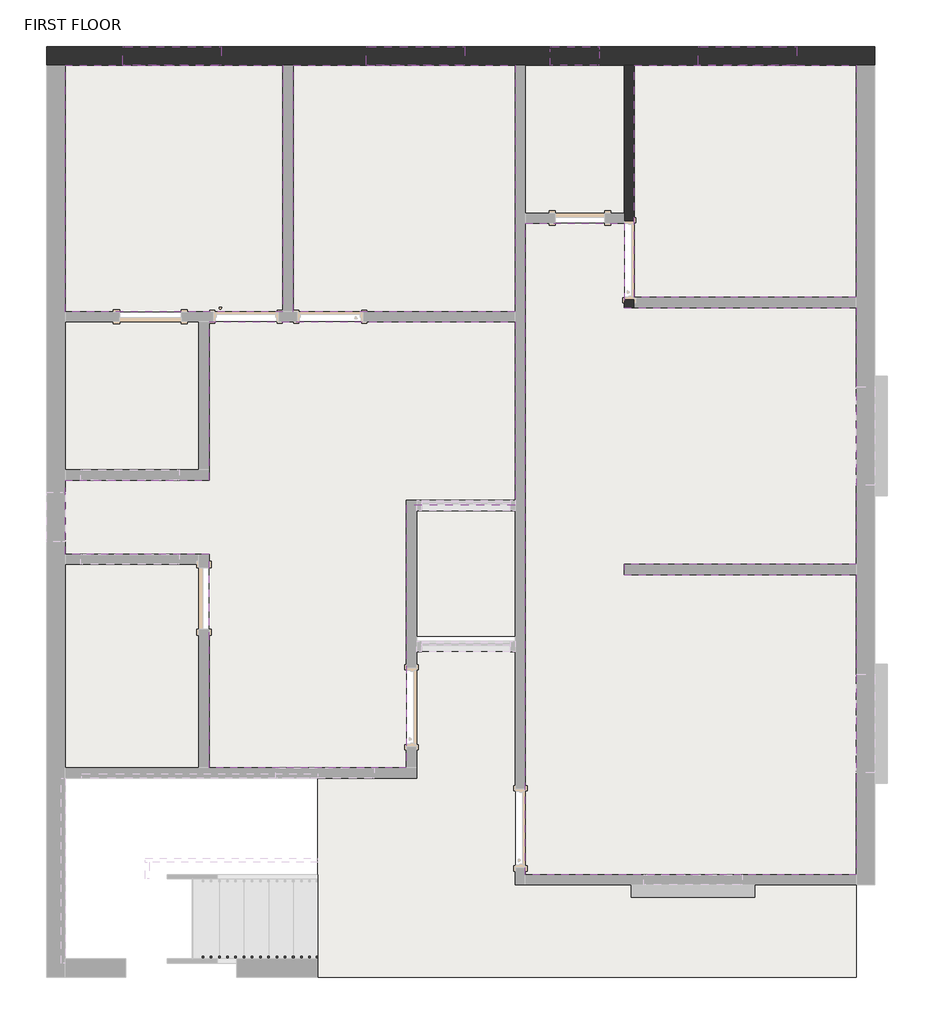
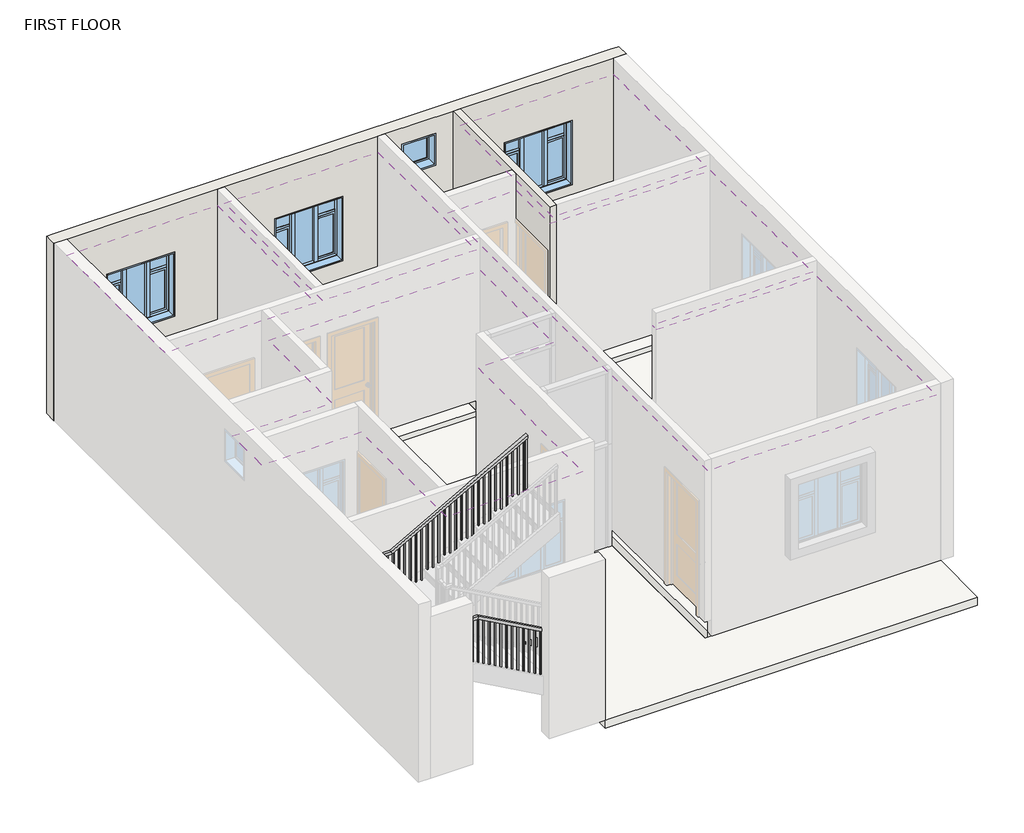
# One storey, part 2 of 3: 5 coverings, 4 windows, 2 walls, 1 railing, 1 slab.
"""IFC4 building model written with IfcOpenShell, lengths in millimetres."""

from ifc_helpers import new_model, si_unit, frame, origin, place, context, project, spatial, polyline, outline, extrude, faceted_brep, transform, mapped, element, save
from components import fixed_opening_window_2_x_2_e119d648, window_casement_triple_side_transom_window_4_x_4_fd24aed3

model = new_model("IFC4")

# Units and contexts
model_context = context("Model", 3, world=origin())
ifc_project = project(units=[si_unit("LENGTHUNIT", "METRE", prefix="MILLI")], contexts=[model_context])

# Site, building, storey
site = spatial("IfcSite", under=ifc_project)
building = spatial("IfcBuilding", under=site)
storey = spatial("IfcBuildingStorey", under=building, Name="FIRST FLOOR", Elevation=3352.8)

# Coverings
placement = place(None, origin())
element("IfcCovering", 1, ObjectType="GWB on Mtl. Stud 2", at=placement, inside=storey, context=model_context, shape_type="SweptSolid", body=[
    extrude(outline(polyline([(-14760.7023867, 8292.2500137), (-12068.3023867, 8292.2500137), (-12068.3023867, 5244.2500137), (-14760.7023867, 5244.2500137), (-14760.7023867, 8292.2500137)])), frame((0.0, 0.0, 6400.8), z_axis=(0.0, 0.0, 1.0), x_axis=(1.0, 0.0, 0.0)), (0.0, 0.0, 1.0), 107.95),
])
element("IfcCovering", 2, ObjectType="GWB on Mtl. Stud 2", at=placement, inside=storey, context=model_context, shape_type="SweptSolid", body=[
    extrude(outline(polyline([(-11941.3023867, 5244.2500137), (-11941.3023867, 8292.2500137), (-9198.1023867, 8292.2500137), (-9198.1023867, 5244.2500137), (-11941.3023867, 5244.2500137)])), frame((0.0, 0.0, 6400.8), z_axis=(0.0, 0.0, 1.0), x_axis=(1.0, 0.0, 0.0)), (0.0, 0.0, 1.0), 107.95),
])
element("IfcCovering", 3, ObjectType="GWB on Mtl. Stud 2", at=placement, inside=storey, context=model_context, shape_type="SweptSolid", body=[
    extrude(outline(polyline([(-7724.9023867, 5422.0500137), (-7724.9023867, 8292.2500137), (-4981.7023867, 8292.2500137), (-4981.7023867, 5422.0500137), (-7724.9023867, 5422.0500137)])), frame((0.0, 0.0, 6400.8), z_axis=(0.0, 0.0, 1.0), x_axis=(1.0, 0.0, 0.0)), (0.0, 0.0, 1.0), 107.95),
])
element("IfcCovering", 4, ObjectType="GWB on Mtl. Stud 2", at=placement, inside=storey, context=model_context, shape_type="SweptSolid", body=[
    extrude(outline(polyline([(-7851.9023867, 5295.0500137), (-4981.7023867, 5295.0500137), (-4981.7023867, 2120.0500137), (-7851.9023867, 2120.0500137), (-7851.9023867, 1993.0500137), (-4981.7023867, 1993.0500137), (-4981.7023867, -1715.3499863), (-9071.1023867, -1715.3499863), (-9071.1023867, 6336.4500137), (-7851.9023867, 6336.4500137), (-7851.9023867, 5295.0500137)])), frame((0.0, 0.0, 6400.8), z_axis=(0.0, 0.0, 1.0), x_axis=(1.0, 0.0, 0.0)), (0.0, 0.0, 1.0), 107.95),
])
element("IfcCovering", 5, ObjectType="GWB on Mtl. Stud 2", at=placement, inside=storey, context=model_context, shape_type="SweptSolid", body=[
    extrude(outline(polyline([(-12982.7023867, 2246.6265627), (-14760.7023867, 2246.6265627), (-14760.7023867, 3161.4500137), (-12982.7023867, 3161.4500137), (-12982.7023867, 5117.2500137), (-9198.1023867, 5117.2500137), (-9198.1023867, 2848.1833471), (-10544.3023867, 2848.1833471), (-10544.3023867, -394.5499863), (-12982.7023867, -394.5499863), (-12982.7023867, 2246.6265627)])), frame((0.0, 0.0, 6096.0), z_axis=(0.0, 0.0, 1.0), x_axis=(1.0, 0.0, 0.0)), (0.0, 0.0, 1.0), 107.95),
])

# Railing
element("IfcRailing", 6, ObjectType="Handrail - Rectangular", at=placement, inside=storey, context=model_context, shape_type="SolidModel", body=[
    faceted_brep([(-11636.5023867, -2756.7499863, 4741.3333333), (-11636.5023867, -2756.7499863, 4683.220221), (-11636.5023867, -2705.9499863, 4683.220221), (-11636.5023867, -2705.9499863, 4741.3333333), (-13770.1023867, -2756.7499863, 5926.6666667), (-13783.2659889, -2756.7499863, 5875.8666667), (-13783.2659889, -2705.9499863, 5875.8666667), (-13770.1023867, -2705.9499863, 5926.6666667), (-14760.7023867, -2756.7499863, 5926.6666667), (-14760.7023867, -2756.7499863, 5875.8666667), (-14709.9023867, -2705.9499863, 5875.8666667), (-14709.9023867, -2705.9499863, 5926.6666667), (-14760.7023867, -521.5499863, 5926.6666667), (-14760.7023867, -521.5499863, 5875.8666667), (-14709.9023867, -572.3499863, 5875.8666667), (-14709.9023867, -572.3499863, 5926.6666667), (-14074.9023867, -521.5499863, 5926.6666667), (-14061.7387844, -521.5499863, 5875.8666667), (-14061.7387844, -572.3499863, 5875.8666667), (-14074.9023867, -572.3499863, 5926.6666667), (-11636.5023867, -521.5499863, 7281.3333333), (-11636.5023867, -572.3499863, 7281.3333333), (-11636.5023867, -572.3499863, 7223.220221), (-11636.5023867, -521.5499863, 7223.220221)], [[[0, 1, 2, 3]], [[1, 0, 4, 5]], [[2, 1, 5, 6]], [[3, 2, 6, 7]], [[0, 3, 7, 4]], [[5, 4, 8, 9]], [[6, 5, 9, 10]], [[7, 6, 10, 11]], [[4, 7, 11, 8]], [[9, 8, 12, 13]], [[10, 9, 13, 14]], [[11, 10, 14, 15]], [[8, 11, 15, 12]], [[13, 12, 16, 17]], [[14, 13, 17, 18]], [[15, 14, 18, 19]], [[12, 15, 19, 16]], [[20, 21, 22, 23]], [[17, 16, 20, 23]], [[18, 17, 23, 22]], [[19, 18, 22, 21]], [[16, 19, 21, 20]]]),
    extrude(outline(polyline([(7189.7063321, -11696.8273867), (6197.6, -11696.8273867), (6197.6, -11677.7773867), (7200.2896654, -11677.7773867), (7189.7063321, -11696.8273867)])), frame((0.0, -556.4749863, 0.0), z_axis=(0.0, 1.0, 0.0), x_axis=(0.0, 0.0, 1.0)), (0.0, 0.0, 1.0), 19.05),
    extrude(outline(polyline([(7133.2618876, -11798.4273867), (6197.6, -11798.4273867), (6197.6, -11779.3773867), (7143.845221, -11779.3773867), (7133.2618876, -11798.4273867)])), frame((0.0, -556.4749863, 0.0), z_axis=(0.0, 1.0, 0.0), x_axis=(0.0, 0.0, 1.0)), (0.0, 0.0, 1.0), 19.05),
    extrude(outline(polyline([(7076.8174432, -11900.0273867), (6197.6, -11900.0273867), (6197.6, -11880.9773867), (7087.4007765, -11880.9773867), (7076.8174432, -11900.0273867)])), frame((0.0, -556.4749863, 0.0), z_axis=(0.0, 1.0, 0.0), x_axis=(0.0, 0.0, 1.0)), (0.0, 0.0, 1.0), 19.05),
    extrude(outline(polyline([(7020.3729988, -12001.6273867), (6028.2666667, -12001.6273867), (6028.2666667, -11982.5773867), (7030.9563321, -11982.5773867), (7020.3729988, -12001.6273867)])), frame((0.0, -556.4749863, 0.0), z_axis=(0.0, 1.0, 0.0), x_axis=(0.0, 0.0, 1.0)), (0.0, 0.0, 1.0), 19.05),
    extrude(outline(polyline([(6963.9285543, -12103.2273867), (6028.2666667, -12103.2273867), (6028.2666667, -12084.1773867), (6974.5118876, -12084.1773867), (6963.9285543, -12103.2273867)])), frame((0.0, -556.4749863, 0.0), z_axis=(0.0, 1.0, 0.0), x_axis=(0.0, 0.0, 1.0)), (0.0, 0.0, 1.0), 19.05),
    extrude(outline(polyline([(6907.4841099, -12204.8273867), (6028.2666667, -12204.8273867), (6028.2666667, -12185.7773867), (6918.0674432, -12185.7773867), (6907.4841099, -12204.8273867)])), frame((0.0, -556.4749863, 0.0), z_axis=(0.0, 1.0, 0.0), x_axis=(0.0, 0.0, 1.0)), (0.0, 0.0, 1.0), 19.05),
    extrude(outline(polyline([(6851.0396654, -12306.4273867), (5858.9333333, -12306.4273867), (5858.9333333, -12287.3773867), (6861.6229988, -12287.3773867), (6851.0396654, -12306.4273867)])), frame((0.0, -556.4749863, 0.0), z_axis=(0.0, 1.0, 0.0), x_axis=(0.0, 0.0, 1.0)), (0.0, 0.0, 1.0), 19.05),
    extrude(outline(polyline([(6794.595221, -12408.0273867), (5858.9333333, -12408.0273867), (5858.9333333, -12388.9773867), (6805.1785543, -12388.9773867), (6794.595221, -12408.0273867)])), frame((0.0, -556.4749863, 0.0), z_axis=(0.0, 1.0, 0.0), x_axis=(0.0, 0.0, 1.0)), (0.0, 0.0, 1.0), 19.05),
    extrude(outline(polyline([(6738.1507765, -12509.6273867), (5858.9333333, -12509.6273867), (5858.9333333, -12490.5773867), (6748.7341099, -12490.5773867), (6738.1507765, -12509.6273867)])), frame((0.0, -556.4749863, 0.0), z_axis=(0.0, 1.0, 0.0), x_axis=(0.0, 0.0, 1.0)), (0.0, 0.0, 1.0), 19.05),
    extrude(outline(polyline([(6681.7063321, -12611.2273867), (5689.6, -12611.2273867), (5689.6, -12592.1773867), (6692.2896654, -12592.1773867), (6681.7063321, -12611.2273867)])), frame((0.0, -556.4749863, 0.0), z_axis=(0.0, 1.0, 0.0), x_axis=(0.0, 0.0, 1.0)), (0.0, 0.0, 1.0), 19.05),
    extrude(outline(polyline([(6625.2618876, -12712.8273867), (5689.6, -12712.8273867), (5689.6, -12693.7773867), (6635.845221, -12693.7773867), (6625.2618876, -12712.8273867)])), frame((0.0, -556.4749863, 0.0), z_axis=(0.0, 1.0, 0.0), x_axis=(0.0, 0.0, 1.0)), (0.0, 0.0, 1.0), 19.05),
    extrude(outline(polyline([(6568.8174432, -12814.4273867), (5689.6, -12814.4273867), (5689.6, -12795.3773867), (6579.4007765, -12795.3773867), (6568.8174432, -12814.4273867)])), frame((0.0, -556.4749863, 0.0), z_axis=(0.0, 1.0, 0.0), x_axis=(0.0, 0.0, 1.0)), (0.0, 0.0, 1.0), 19.05),
    extrude(outline(polyline([(6512.3729988, -12916.0273867), (5520.2666667, -12916.0273867), (5520.2666667, -12896.9773867), (6522.9563321, -12896.9773867), (6512.3729988, -12916.0273867)])), frame((0.0, -556.4749863, 0.0), z_axis=(0.0, 1.0, 0.0), x_axis=(0.0, 0.0, 1.0)), (0.0, 0.0, 1.0), 19.05),
    extrude(outline(polyline([(6455.9285543, -13017.6273867), (5520.2666667, -13017.6273867), (5520.2666667, -12998.5773867), (6466.5118876, -12998.5773867), (6455.9285543, -13017.6273867)])), frame((0.0, -556.4749863, 0.0), z_axis=(0.0, 1.0, 0.0), x_axis=(0.0, 0.0, 1.0)), (0.0, 0.0, 1.0), 19.05),
    extrude(outline(polyline([(6399.4841099, -13119.2273867), (5520.2666667, -13119.2273867), (5520.2666667, -13100.1773867), (6410.0674432, -13100.1773867), (6399.4841099, -13119.2273867)])), frame((0.0, -556.4749863, 0.0), z_axis=(0.0, 1.0, 0.0), x_axis=(0.0, 0.0, 1.0)), (0.0, 0.0, 1.0), 19.05),
    extrude(outline(polyline([(6343.0396654, -13220.8273867), (5350.9333333, -13220.8273867), (5350.9333333, -13201.7773867), (6353.6229988, -13201.7773867), (6343.0396654, -13220.8273867)])), frame((0.0, -556.4749863, 0.0), z_axis=(0.0, 1.0, 0.0), x_axis=(0.0, 0.0, 1.0)), (0.0, 0.0, 1.0), 19.05),
    extrude(outline(polyline([(6286.595221, -13322.4273867), (5350.9333333, -13322.4273867), (5350.9333333, -13303.3773867), (6297.1785543, -13303.3773867), (6286.595221, -13322.4273867)])), frame((0.0, -556.4749863, 0.0), z_axis=(0.0, 1.0, 0.0), x_axis=(0.0, 0.0, 1.0)), (0.0, 0.0, 1.0), 19.05),
    extrude(outline(polyline([(6230.1507765, -13424.0273867), (5350.9333333, -13424.0273867), (5350.9333333, -13404.9773867), (6240.7341099, -13404.9773867), (6230.1507765, -13424.0273867)])), frame((0.0, -556.4749863, 0.0), z_axis=(0.0, 1.0, 0.0), x_axis=(0.0, 0.0, 1.0)), (0.0, 0.0, 1.0), 19.05),
    extrude(outline(polyline([(6173.7063321, -13525.6273867), (5181.6, -13525.6273867), (5181.6, -13506.5773867), (6184.2896654, -13506.5773867), (6173.7063321, -13525.6273867)])), frame((0.0, -556.4749863, 0.0), z_axis=(0.0, 1.0, 0.0), x_axis=(0.0, 0.0, 1.0)), (0.0, 0.0, 1.0), 19.05),
    extrude(outline(polyline([(6117.2618876, -13627.2273867), (5181.6, -13627.2273867), (5181.6, -13608.1773867), (6127.845221, -13608.1773867), (6117.2618876, -13627.2273867)])), frame((0.0, -556.4749863, 0.0), z_axis=(0.0, 1.0, 0.0), x_axis=(0.0, 0.0, 1.0)), (0.0, 0.0, 1.0), 19.05),
    extrude(outline(polyline([(6060.8174432, -13728.8273867), (5181.6, -13728.8273867), (5181.6, -13709.7773867), (6071.4007765, -13709.7773867), (6060.8174432, -13728.8273867)])), frame((0.0, -556.4749863, 0.0), z_axis=(0.0, 1.0, 0.0), x_axis=(0.0, 0.0, 1.0)), (0.0, 0.0, 1.0), 19.05),
    extrude(outline(polyline([(6004.3729988, -13830.4273867), (5012.2666667, -13830.4273867), (5012.2666667, -13811.3773867), (6014.9563321, -13811.3773867), (6004.3729988, -13830.4273867)])), frame((0.0, -556.4749863, 0.0), z_axis=(0.0, 1.0, 0.0), x_axis=(0.0, 0.0, 1.0)), (0.0, 0.0, 1.0), 19.05),
    extrude(outline(polyline([(5947.9285543, -13932.0273867), (5012.2666667, -13932.0273867), (5012.2666667, -13912.9773867), (5958.5118876, -13912.9773867), (5947.9285543, -13932.0273867)])), frame((0.0, -556.4749863, 0.0), z_axis=(0.0, 1.0, 0.0), x_axis=(0.0, 0.0, 1.0)), (0.0, 0.0, 1.0), 19.05),
    extrude(outline(polyline([(5891.4841099, -14033.6273867), (5012.2666667, -14033.6273867), (5012.2666667, -14014.5773867), (5902.0674432, -14014.5773867), (5891.4841099, -14033.6273867)])), frame((0.0, -556.4749863, 0.0), z_axis=(0.0, 1.0, 0.0), x_axis=(0.0, 0.0, 1.0)), (0.0, 0.0, 1.0), 19.05),
    extrude(outline(polyline([(-14135.2273867, -537.4249863), (-14116.1773867, -537.4249863), (-14116.1773867, -556.4749863), (-14135.2273867, -556.4749863), (-14135.2273867, -537.4249863)])), frame((0.0, 0.0, 5012.2666667), z_axis=(0.0, 0.0, 1.0), x_axis=(1.0, 0.0, 0.0)), (0.0, 0.0, 1.0), 863.6),
    extrude(outline(polyline([(-14236.8273867, -537.4249863), (-14217.7773867, -537.4249863), (-14217.7773867, -556.4749863), (-14236.8273867, -556.4749863), (-14236.8273867, -537.4249863)])), frame((0.0, 0.0, 5012.2666667), z_axis=(0.0, 0.0, 1.0), x_axis=(1.0, 0.0, 0.0)), (0.0, 0.0, 1.0), 863.6),
    extrude(outline(polyline([(-14338.4273867, -537.4249863), (-14319.3773867, -537.4249863), (-14319.3773867, -556.4749863), (-14338.4273867, -556.4749863), (-14338.4273867, -537.4249863)])), frame((0.0, 0.0, 5012.2666667), z_axis=(0.0, 0.0, 1.0), x_axis=(1.0, 0.0, 0.0)), (0.0, 0.0, 1.0), 863.6),
    extrude(outline(polyline([(-14440.0273867, -537.4249863), (-14420.9773867, -537.4249863), (-14420.9773867, -556.4749863), (-14440.0273867, -556.4749863), (-14440.0273867, -537.4249863)])), frame((0.0, 0.0, 5012.2666667), z_axis=(0.0, 0.0, 1.0), x_axis=(1.0, 0.0, 0.0)), (0.0, 0.0, 1.0), 863.6),
    extrude(outline(polyline([(-14541.6273867, -537.4249863), (-14522.5773867, -537.4249863), (-14522.5773867, -556.4749863), (-14541.6273867, -556.4749863), (-14541.6273867, -537.4249863)])), frame((0.0, 0.0, 5012.2666667), z_axis=(0.0, 0.0, 1.0), x_axis=(1.0, 0.0, 0.0)), (0.0, 0.0, 1.0), 863.6),
    extrude(outline(polyline([(-14643.2273867, -537.4249863), (-14624.1773867, -537.4249863), (-14624.1773867, -556.4749863), (-14643.2273867, -556.4749863), (-14643.2273867, -537.4249863)])), frame((0.0, 0.0, 5012.2666667), z_axis=(0.0, 0.0, 1.0), x_axis=(1.0, 0.0, 0.0)), (0.0, 0.0, 1.0), 863.6),
    extrude(outline(polyline([(-14744.8273867, -607.2749863), (-14744.8273867, -588.2249863), (-14725.7773867, -588.2249863), (-14725.7773867, -607.2749863), (-14744.8273867, -607.2749863)])), frame((0.0, 0.0, 5012.2666667), z_axis=(0.0, 0.0, 1.0), x_axis=(1.0, 0.0, 0.0)), (0.0, 0.0, 1.0), 863.6),
    extrude(outline(polyline([(-14744.8273867, -708.8749863), (-14744.8273867, -689.8249863), (-14725.7773867, -689.8249863), (-14725.7773867, -708.8749863), (-14744.8273867, -708.8749863)])), frame((0.0, 0.0, 5012.2666667), z_axis=(0.0, 0.0, 1.0), x_axis=(1.0, 0.0, 0.0)), (0.0, 0.0, 1.0), 863.6),
    extrude(outline(polyline([(-14744.8273867, -810.4749863), (-14744.8273867, -791.4249863), (-14725.7773867, -791.4249863), (-14725.7773867, -810.4749863), (-14744.8273867, -810.4749863)])), frame((0.0, 0.0, 5012.2666667), z_axis=(0.0, 0.0, 1.0), x_axis=(1.0, 0.0, 0.0)), (0.0, 0.0, 1.0), 863.6),
    extrude(outline(polyline([(-14744.8273867, -912.0749863), (-14744.8273867, -893.0249863), (-14725.7773867, -893.0249863), (-14725.7773867, -912.0749863), (-14744.8273867, -912.0749863)])), frame((0.0, 0.0, 5012.2666667), z_axis=(0.0, 0.0, 1.0), x_axis=(1.0, 0.0, 0.0)), (0.0, 0.0, 1.0), 863.6),
    extrude(outline(polyline([(-14744.8273867, -1013.6749863), (-14744.8273867, -994.6249863), (-14725.7773867, -994.6249863), (-14725.7773867, -1013.6749863), (-14744.8273867, -1013.6749863)])), frame((0.0, 0.0, 5012.2666667), z_axis=(0.0, 0.0, 1.0), x_axis=(1.0, 0.0, 0.0)), (0.0, 0.0, 1.0), 863.6),
    extrude(outline(polyline([(-14744.8273867, -1115.2749863), (-14744.8273867, -1096.2249863), (-14725.7773867, -1096.2249863), (-14725.7773867, -1115.2749863), (-14744.8273867, -1115.2749863)])), frame((0.0, 0.0, 5012.2666667), z_axis=(0.0, 0.0, 1.0), x_axis=(1.0, 0.0, 0.0)), (0.0, 0.0, 1.0), 863.6),
    extrude(outline(polyline([(-14744.8273867, -1216.8749863), (-14744.8273867, -1197.8249863), (-14725.7773867, -1197.8249863), (-14725.7773867, -1216.8749863), (-14744.8273867, -1216.8749863)])), frame((0.0, 0.0, 5012.2666667), z_axis=(0.0, 0.0, 1.0), x_axis=(1.0, 0.0, 0.0)), (0.0, 0.0, 1.0), 863.6),
    extrude(outline(polyline([(-14744.8273867, -1318.4749863), (-14744.8273867, -1299.4249863), (-14725.7773867, -1299.4249863), (-14725.7773867, -1318.4749863), (-14744.8273867, -1318.4749863)])), frame((0.0, 0.0, 5012.2666667), z_axis=(0.0, 0.0, 1.0), x_axis=(1.0, 0.0, 0.0)), (0.0, 0.0, 1.0), 863.6),
    extrude(outline(polyline([(-14744.8273867, -1420.0749863), (-14744.8273867, -1401.0249863), (-14725.7773867, -1401.0249863), (-14725.7773867, -1420.0749863), (-14744.8273867, -1420.0749863)])), frame((0.0, 0.0, 5012.2666667), z_axis=(0.0, 0.0, 1.0), x_axis=(1.0, 0.0, 0.0)), (0.0, 0.0, 1.0), 863.6),
    extrude(outline(polyline([(-14744.8273867, -1521.6749863), (-14744.8273867, -1502.6249863), (-14725.7773867, -1502.6249863), (-14725.7773867, -1521.6749863), (-14744.8273867, -1521.6749863)])), frame((0.0, 0.0, 5012.2666667), z_axis=(0.0, 0.0, 1.0), x_axis=(1.0, 0.0, 0.0)), (0.0, 0.0, 1.0), 863.6),
    extrude(outline(polyline([(-14744.8273867, -1623.2749863), (-14744.8273867, -1604.2249863), (-14725.7773867, -1604.2249863), (-14725.7773867, -1623.2749863), (-14744.8273867, -1623.2749863)])), frame((0.0, 0.0, 5012.2666667), z_axis=(0.0, 0.0, 1.0), x_axis=(1.0, 0.0, 0.0)), (0.0, 0.0, 1.0), 863.6),
    extrude(outline(polyline([(-14744.8273867, -1724.8749863), (-14744.8273867, -1705.8249863), (-14725.7773867, -1705.8249863), (-14725.7773867, -1724.8749863), (-14744.8273867, -1724.8749863)])), frame((0.0, 0.0, 5012.2666667), z_axis=(0.0, 0.0, 1.0), x_axis=(1.0, 0.0, 0.0)), (0.0, 0.0, 1.0), 863.6),
    extrude(outline(polyline([(-14744.8273867, -1826.4749863), (-14744.8273867, -1807.4249863), (-14725.7773867, -1807.4249863), (-14725.7773867, -1826.4749863), (-14744.8273867, -1826.4749863)])), frame((0.0, 0.0, 5012.2666667), z_axis=(0.0, 0.0, 1.0), x_axis=(1.0, 0.0, 0.0)), (0.0, 0.0, 1.0), 863.6),
    extrude(outline(polyline([(-14744.8273867, -1928.0749863), (-14744.8273867, -1909.0249863), (-14725.7773867, -1909.0249863), (-14725.7773867, -1928.0749863), (-14744.8273867, -1928.0749863)])), frame((0.0, 0.0, 5012.2666667), z_axis=(0.0, 0.0, 1.0), x_axis=(1.0, 0.0, 0.0)), (0.0, 0.0, 1.0), 863.6),
    extrude(outline(polyline([(-14744.8273867, -2029.6749863), (-14744.8273867, -2010.6249863), (-14725.7773867, -2010.6249863), (-14725.7773867, -2029.6749863), (-14744.8273867, -2029.6749863)])), frame((0.0, 0.0, 5012.2666667), z_axis=(0.0, 0.0, 1.0), x_axis=(1.0, 0.0, 0.0)), (0.0, 0.0, 1.0), 863.6),
    extrude(outline(polyline([(-14744.8273867, -2131.2749863), (-14744.8273867, -2112.2249863), (-14725.7773867, -2112.2249863), (-14725.7773867, -2131.2749863), (-14744.8273867, -2131.2749863)])), frame((0.0, 0.0, 5012.2666667), z_axis=(0.0, 0.0, 1.0), x_axis=(1.0, 0.0, 0.0)), (0.0, 0.0, 1.0), 863.6),
    extrude(outline(polyline([(-14744.8273867, -2232.8749863), (-14744.8273867, -2213.8249863), (-14725.7773867, -2213.8249863), (-14725.7773867, -2232.8749863), (-14744.8273867, -2232.8749863)])), frame((0.0, 0.0, 5012.2666667), z_axis=(0.0, 0.0, 1.0), x_axis=(1.0, 0.0, 0.0)), (0.0, 0.0, 1.0), 863.6),
    extrude(outline(polyline([(-14744.8273867, -2334.4749863), (-14744.8273867, -2315.4249863), (-14725.7773867, -2315.4249863), (-14725.7773867, -2334.4749863), (-14744.8273867, -2334.4749863)])), frame((0.0, 0.0, 5012.2666667), z_axis=(0.0, 0.0, 1.0), x_axis=(1.0, 0.0, 0.0)), (0.0, 0.0, 1.0), 863.6),
    extrude(outline(polyline([(-14744.8273867, -2436.0749863), (-14744.8273867, -2417.0249863), (-14725.7773867, -2417.0249863), (-14725.7773867, -2436.0749863), (-14744.8273867, -2436.0749863)])), frame((0.0, 0.0, 5012.2666667), z_axis=(0.0, 0.0, 1.0), x_axis=(1.0, 0.0, 0.0)), (0.0, 0.0, 1.0), 863.6),
    extrude(outline(polyline([(-14744.8273867, -2537.6749863), (-14744.8273867, -2518.6249863), (-14725.7773867, -2518.6249863), (-14725.7773867, -2537.6749863), (-14744.8273867, -2537.6749863)])), frame((0.0, 0.0, 5012.2666667), z_axis=(0.0, 0.0, 1.0), x_axis=(1.0, 0.0, 0.0)), (0.0, 0.0, 1.0), 863.6),
    extrude(outline(polyline([(-14744.8273867, -2639.2749863), (-14744.8273867, -2620.2249863), (-14725.7773867, -2620.2249863), (-14725.7773867, -2639.2749863), (-14744.8273867, -2639.2749863)])), frame((0.0, 0.0, 5012.2666667), z_axis=(0.0, 0.0, 1.0), x_axis=(1.0, 0.0, 0.0)), (0.0, 0.0, 1.0), 863.6),
    extrude(outline(polyline([(-14674.9773867, -2740.8749863), (-14694.0273867, -2740.8749863), (-14694.0273867, -2721.8249863), (-14674.9773867, -2721.8249863), (-14674.9773867, -2740.8749863)])), frame((0.0, 0.0, 5012.2666667), z_axis=(0.0, 0.0, 1.0), x_axis=(1.0, 0.0, 0.0)), (0.0, 0.0, 1.0), 863.6),
    extrude(outline(polyline([(-14573.3773867, -2740.8749863), (-14592.4273867, -2740.8749863), (-14592.4273867, -2721.8249863), (-14573.3773867, -2721.8249863), (-14573.3773867, -2740.8749863)])), frame((0.0, 0.0, 5012.2666667), z_axis=(0.0, 0.0, 1.0), x_axis=(1.0, 0.0, 0.0)), (0.0, 0.0, 1.0), 863.6),
    extrude(outline(polyline([(-14471.7773867, -2740.8749863), (-14490.8273867, -2740.8749863), (-14490.8273867, -2721.8249863), (-14471.7773867, -2721.8249863), (-14471.7773867, -2740.8749863)])), frame((0.0, 0.0, 5012.2666667), z_axis=(0.0, 0.0, 1.0), x_axis=(1.0, 0.0, 0.0)), (0.0, 0.0, 1.0), 863.6),
    extrude(outline(polyline([(-14370.1773867, -2740.8749863), (-14389.2273867, -2740.8749863), (-14389.2273867, -2721.8249863), (-14370.1773867, -2721.8249863), (-14370.1773867, -2740.8749863)])), frame((0.0, 0.0, 5012.2666667), z_axis=(0.0, 0.0, 1.0), x_axis=(1.0, 0.0, 0.0)), (0.0, 0.0, 1.0), 863.6),
    extrude(outline(polyline([(-14268.5773867, -2740.8749863), (-14287.6273867, -2740.8749863), (-14287.6273867, -2721.8249863), (-14268.5773867, -2721.8249863), (-14268.5773867, -2740.8749863)])), frame((0.0, 0.0, 5012.2666667), z_axis=(0.0, 0.0, 1.0), x_axis=(1.0, 0.0, 0.0)), (0.0, 0.0, 1.0), 863.6),
    extrude(outline(polyline([(-14166.9773867, -2740.8749863), (-14186.0273867, -2740.8749863), (-14186.0273867, -2721.8249863), (-14166.9773867, -2721.8249863), (-14166.9773867, -2740.8749863)])), frame((0.0, 0.0, 5012.2666667), z_axis=(0.0, 0.0, 1.0), x_axis=(1.0, 0.0, 0.0)), (0.0, 0.0, 1.0), 863.6),
    extrude(outline(polyline([(-14065.3773867, -2740.8749863), (-14084.4273867, -2740.8749863), (-14084.4273867, -2721.8249863), (-14065.3773867, -2721.8249863), (-14065.3773867, -2740.8749863)])), frame((0.0, 0.0, 5012.2666667), z_axis=(0.0, 0.0, 1.0), x_axis=(1.0, 0.0, 0.0)), (0.0, 0.0, 1.0), 863.6),
    extrude(outline(polyline([(-13963.7773867, -2740.8749863), (-13982.8273867, -2740.8749863), (-13982.8273867, -2721.8249863), (-13963.7773867, -2721.8249863), (-13963.7773867, -2740.8749863)])), frame((0.0, 0.0, 5012.2666667), z_axis=(0.0, 0.0, 1.0), x_axis=(1.0, 0.0, 0.0)), (0.0, 0.0, 1.0), 863.6),
    extrude(outline(polyline([(-13862.1773867, -2740.8749863), (-13881.2273867, -2740.8749863), (-13881.2273867, -2721.8249863), (-13862.1773867, -2721.8249863), (-13862.1773867, -2740.8749863)])), frame((0.0, 0.0, 5012.2666667), z_axis=(0.0, 0.0, 1.0), x_axis=(1.0, 0.0, 0.0)), (0.0, 0.0, 1.0), 863.6),
    extrude(outline(polyline([(5873.845221, -13779.6273867), (5012.2666667, -13779.6273867), (5012.2666667, -13760.5773867), (5863.2618876, -13760.5773867), (5873.845221, -13779.6273867)])), frame((0.0, -2740.8749863, 0.0), z_axis=(0.0, 1.0, 0.0), x_axis=(0.0, 0.0, 1.0)), (0.0, 0.0, 1.0), 19.05),
    extrude(outline(polyline([(5817.4007765, -13678.0273867), (4842.9333333, -13678.0273867), (4842.9333333, -13658.9773867), (5806.8174432, -13658.9773867), (5817.4007765, -13678.0273867)])), frame((0.0, -2740.8749863, 0.0), z_axis=(0.0, 1.0, 0.0), x_axis=(0.0, 0.0, 1.0)), (0.0, 0.0, 1.0), 19.05),
    extrude(outline(polyline([(5760.9563321, -13576.4273867), (4842.9333333, -13576.4273867), (4842.9333333, -13557.3773867), (5750.3729988, -13557.3773867), (5760.9563321, -13576.4273867)])), frame((0.0, -2740.8749863, 0.0), z_axis=(0.0, 1.0, 0.0), x_axis=(0.0, 0.0, 1.0)), (0.0, 0.0, 1.0), 19.05),
    extrude(outline(polyline([(5704.5118876, -13474.8273867), (4842.9333333, -13474.8273867), (4842.9333333, -13455.7773867), (5693.9285543, -13455.7773867), (5704.5118876, -13474.8273867)])), frame((0.0, -2740.8749863, 0.0), z_axis=(0.0, 1.0, 0.0), x_axis=(0.0, 0.0, 1.0)), (0.0, 0.0, 1.0), 19.05),
    extrude(outline(polyline([(5648.0674432, -13373.2273867), (4673.6, -13373.2273867), (4673.6, -13354.1773867), (5637.4841099, -13354.1773867), (5648.0674432, -13373.2273867)])), frame((0.0, -2740.8749863, 0.0), z_axis=(0.0, 1.0, 0.0), x_axis=(0.0, 0.0, 1.0)), (0.0, 0.0, 1.0), 19.05),
    extrude(outline(polyline([(5591.6229988, -13271.6273867), (4673.6, -13271.6273867), (4673.6, -13252.5773867), (5581.0396654, -13252.5773867), (5591.6229988, -13271.6273867)])), frame((0.0, -2740.8749863, 0.0), z_axis=(0.0, 1.0, 0.0), x_axis=(0.0, 0.0, 1.0)), (0.0, 0.0, 1.0), 19.05),
    extrude(outline(polyline([(5535.1785543, -13170.0273867), (4673.6, -13170.0273867), (4673.6, -13150.9773867), (5524.595221, -13150.9773867), (5535.1785543, -13170.0273867)])), frame((0.0, -2740.8749863, 0.0), z_axis=(0.0, 1.0, 0.0), x_axis=(0.0, 0.0, 1.0)), (0.0, 0.0, 1.0), 19.05),
    extrude(outline(polyline([(5478.7341099, -13068.4273867), (4504.2666667, -13068.4273867), (4504.2666667, -13049.3773867), (5468.1507765, -13049.3773867), (5478.7341099, -13068.4273867)])), frame((0.0, -2740.8749863, 0.0), z_axis=(0.0, 1.0, 0.0), x_axis=(0.0, 0.0, 1.0)), (0.0, 0.0, 1.0), 19.05),
    extrude(outline(polyline([(5422.2896654, -12966.8273867), (4504.2666667, -12966.8273867), (4504.2666667, -12947.7773867), (5411.7063321, -12947.7773867), (5422.2896654, -12966.8273867)])), frame((0.0, -2740.8749863, 0.0), z_axis=(0.0, 1.0, 0.0), x_axis=(0.0, 0.0, 1.0)), (0.0, 0.0, 1.0), 19.05),
    extrude(outline(polyline([(5365.845221, -12865.2273867), (4504.2666667, -12865.2273867), (4504.2666667, -12846.1773867), (5355.2618876, -12846.1773867), (5365.845221, -12865.2273867)])), frame((0.0, -2740.8749863, 0.0), z_axis=(0.0, 1.0, 0.0), x_axis=(0.0, 0.0, 1.0)), (0.0, 0.0, 1.0), 19.05),
    extrude(outline(polyline([(5309.4007765, -12763.6273867), (4334.9333333, -12763.6273867), (4334.9333333, -12744.5773867), (5298.8174432, -12744.5773867), (5309.4007765, -12763.6273867)])), frame((0.0, -2740.8749863, 0.0), z_axis=(0.0, 1.0, 0.0), x_axis=(0.0, 0.0, 1.0)), (0.0, 0.0, 1.0), 19.05),
    extrude(outline(polyline([(5252.9563321, -12662.0273867), (4334.9333333, -12662.0273867), (4334.9333333, -12642.9773867), (5242.3729988, -12642.9773867), (5252.9563321, -12662.0273867)])), frame((0.0, -2740.8749863, 0.0), z_axis=(0.0, 1.0, 0.0), x_axis=(0.0, 0.0, 1.0)), (0.0, 0.0, 1.0), 19.05),
    extrude(outline(polyline([(5196.5118876, -12560.4273867), (4334.9333333, -12560.4273867), (4334.9333333, -12541.3773867), (5185.9285543, -12541.3773867), (5196.5118876, -12560.4273867)])), frame((0.0, -2740.8749863, 0.0), z_axis=(0.0, 1.0, 0.0), x_axis=(0.0, 0.0, 1.0)), (0.0, 0.0, 1.0), 19.05),
    extrude(outline(polyline([(5140.0674432, -12458.8273867), (4165.6, -12458.8273867), (4165.6, -12439.7773867), (5129.4841099, -12439.7773867), (5140.0674432, -12458.8273867)])), frame((0.0, -2740.8749863, 0.0), z_axis=(0.0, 1.0, 0.0), x_axis=(0.0, 0.0, 1.0)), (0.0, 0.0, 1.0), 19.05),
    extrude(outline(polyline([(5083.6229988, -12357.2273867), (4165.6, -12357.2273867), (4165.6, -12338.1773867), (5073.0396654, -12338.1773867), (5083.6229988, -12357.2273867)])), frame((0.0, -2740.8749863, 0.0), z_axis=(0.0, 1.0, 0.0), x_axis=(0.0, 0.0, 1.0)), (0.0, 0.0, 1.0), 19.05),
    extrude(outline(polyline([(5027.1785543, -12255.6273867), (4165.6, -12255.6273867), (4165.6, -12236.5773867), (5016.595221, -12236.5773867), (5027.1785543, -12255.6273867)])), frame((0.0, -2740.8749863, 0.0), z_axis=(0.0, 1.0, 0.0), x_axis=(0.0, 0.0, 1.0)), (0.0, 0.0, 1.0), 19.05),
    extrude(outline(polyline([(4970.7341099, -12154.0273867), (3996.2666667, -12154.0273867), (3996.2666667, -12134.9773867), (4960.1507765, -12134.9773867), (4970.7341099, -12154.0273867)])), frame((0.0, -2740.8749863, 0.0), z_axis=(0.0, 1.0, 0.0), x_axis=(0.0, 0.0, 1.0)), (0.0, 0.0, 1.0), 19.05),
    extrude(outline(polyline([(4914.2896654, -12052.4273867), (3996.2666667, -12052.4273867), (3996.2666667, -12033.3773867), (4903.7063321, -12033.3773867), (4914.2896654, -12052.4273867)])), frame((0.0, -2740.8749863, 0.0), z_axis=(0.0, 1.0, 0.0), x_axis=(0.0, 0.0, 1.0)), (0.0, 0.0, 1.0), 19.05),
    extrude(outline(polyline([(4857.845221, -11950.8273867), (3996.2666667, -11950.8273867), (3996.2666667, -11931.7773867), (4847.2618876, -11931.7773867), (4857.845221, -11950.8273867)])), frame((0.0, -2740.8749863, 0.0), z_axis=(0.0, 1.0, 0.0), x_axis=(0.0, 0.0, 1.0)), (0.0, 0.0, 1.0), 19.05),
    extrude(outline(polyline([(4801.4007765, -11849.2273867), (3826.9333333, -11849.2273867), (3826.9333333, -11830.1773867), (4790.8174432, -11830.1773867), (4801.4007765, -11849.2273867)])), frame((0.0, -2740.8749863, 0.0), z_axis=(0.0, 1.0, 0.0), x_axis=(0.0, 0.0, 1.0)), (0.0, 0.0, 1.0), 19.05),
    extrude(outline(polyline([(4744.9563321, -11747.6273867), (3826.9333333, -11747.6273867), (3826.9333333, -11728.5773867), (4734.3729988, -11728.5773867), (4744.9563321, -11747.6273867)])), frame((0.0, -2740.8749863, 0.0), z_axis=(0.0, 1.0, 0.0), x_axis=(0.0, 0.0, 1.0)), (0.0, 0.0, 1.0), 19.05),
    extrude(outline(polyline([(-14744.8273867, -556.4749863), (-14744.8273867, -537.4249863), (-14725.7773867, -537.4249863), (-14725.7773867, -556.4749863), (-14744.8273867, -556.4749863)])), frame((0.0, 0.0, 5012.2666667), z_axis=(0.0, 0.0, 1.0), x_axis=(1.0, 0.0, 0.0)), (0.0, 0.0, 1.0), 863.6),
    extrude(outline(polyline([(-14725.7773867, -2740.8749863), (-14744.8273867, -2740.8749863), (-14744.8273867, -2721.8249863), (-14725.7773867, -2721.8249863), (-14725.7773867, -2740.8749863)])), frame((0.0, 0.0, 5012.2666667), z_axis=(0.0, 0.0, 1.0), x_axis=(1.0, 0.0, 0.0)), (0.0, 0.0, 1.0), 863.6),
    extrude(outline(polyline([(7212.6368876, -11655.5523867), (6197.6, -11655.5523867), (6197.6, -11636.5023867), (7223.220221, -11636.5023867), (7212.6368876, -11655.5523867)])), frame((0.0, -556.4749863, 0.0), z_axis=(0.0, 1.0, 0.0), x_axis=(0.0, 0.0, 1.0)), (0.0, 0.0, 1.0), 19.05),
    extrude(outline(polyline([(4693.8035543, -11655.5523867), (3826.9333333, -11655.5523867), (3826.9333333, -11636.5023867), (4683.220221, -11636.5023867), (4693.8035543, -11655.5523867)])), frame((0.0, -2740.8749863, 0.0), z_axis=(0.0, 1.0, 0.0), x_axis=(0.0, 0.0, 1.0)), (0.0, 0.0, 1.0), 19.05),
])

# Slab
element("IfcSlab", 7, ObjectType="marble 6\"", at=placement, inside=storey, context=model_context, shape_type="SweptSolid", body=[
    extrude(outline(polyline([(-12074.6523867, 8292.2500137), (-12074.6523867, 5244.2500137), (-14760.7023867, 5244.2500137), (-14760.7023867, 8292.2500137), (-12074.6523867, 8292.2500137)])), frame((0.0, 0.0, 3200.4), z_axis=(0.0, 0.0, 1.0), x_axis=(1.0, 0.0, 0.0)), (0.0, 0.0, 1.0), 152.4),
    extrude(outline(polyline([(-9198.1023867, 8292.2500137), (-9198.1023867, 5244.2500137), (-11941.3023867, 5244.2500137), (-11941.3023867, 8292.2500137), (-9198.1023867, 8292.2500137)])), frame((0.0, 0.0, 3200.4), z_axis=(0.0, 0.0, 1.0), x_axis=(1.0, 0.0, 0.0)), (0.0, 0.0, 1.0), 152.4),
    extrude(outline(polyline([(-4981.7023867, 8292.2500137), (-4981.7023867, 5422.0500137), (-7724.9023867, 5422.0500137), (-7724.9023867, 8292.2500137), (-4981.7023867, 8292.2500137)])), frame((0.0, 0.0, 3200.4), z_axis=(0.0, 0.0, 1.0), x_axis=(1.0, 0.0, 0.0)), (0.0, 0.0, 1.0), 152.4),
    extrude(outline(polyline([(-7851.9023867, 8292.2500137), (-7851.9023867, 6463.4500137), (-9071.1023867, 6463.4500137), (-9071.1023867, 8292.2500137), (-7851.9023867, 8292.2500137)])), frame((0.0, 0.0, 3200.4), z_axis=(0.0, 0.0, 1.0), x_axis=(1.0, 0.0, 0.0)), (0.0, 0.0, 1.0), 152.4),
    extrude(outline(polyline([(-13109.7023867, 5117.2500137), (-13109.7023867, 3288.4500137), (-14760.7023867, 3288.4500137), (-14760.7023867, 5117.2500137), (-13109.7023867, 5117.2500137)])), frame((0.0, 0.0, 3200.4), z_axis=(0.0, 0.0, 1.0), x_axis=(1.0, 0.0, 0.0)), (0.0, 0.0, 1.0), 152.4),
    extrude(outline(polyline([(-10544.3023867, -394.5499863), (-12982.7023867, -394.5499863), (-12982.7023867, 2246.6265627), (-14760.7023867, 2246.6265627), (-14760.7023867, 3161.4500137), (-12982.7023867, 3161.4500137), (-12982.7023867, 5117.2500137), (-9198.1023867, 5117.2500137), (-9198.1023867, 2911.6833471), (-10544.3023867, 2911.6833471), (-10544.3023867, -394.5499863)])), frame((0.0, 0.0, 3200.4), z_axis=(0.0, 0.0, 1.0), x_axis=(1.0, 0.0, 0.0)), (0.0, 0.0, 1.0), 152.4),
    extrude(outline(polyline([(-13109.7023867, 2119.6265627), (-13109.7023867, -394.5499863), (-14760.7023867, -394.5499863), (-14760.7023867, 2119.6265627), (-13109.7023867, 2119.6265627)])), frame((0.0, 0.0, 3200.4), z_axis=(0.0, 0.0, 1.0), x_axis=(1.0, 0.0, 0.0)), (0.0, 0.0, 1.0), 152.4),
    extrude(outline(polyline([(-9198.1023867, 1231.0500137), (-10417.3023867, 1231.0500137), (-10417.3023867, 2784.6833471), (-9198.1023867, 2784.6833471), (-9198.1023867, 1231.0500137)])), frame((0.0, 0.0, 3200.4), z_axis=(0.0, 0.0, 1.0), x_axis=(1.0, 0.0, 0.0)), (0.0, 0.0, 1.0), 152.4),
    extrude(outline(polyline([(-4981.7023867, -1715.3499863), (-9071.1023867, -1715.3499863), (-9071.1023867, 6336.4500137), (-7851.9023867, 6336.4500137), (-7851.9023867, 5295.0500137), (-4981.7023867, 5295.0500137), (-4981.7023867, 2120.0500137), (-7851.9023867, 2120.0500137), (-7851.9023867, 1993.0500137), (-4981.7023867, 1993.0500137), (-4981.7023867, -1715.3499863)])), frame((0.0, 0.0, 3200.4), z_axis=(0.0, 0.0, 1.0), x_axis=(1.0, 0.0, 0.0)), (0.0, 0.0, 1.0), 152.4),
    extrude(outline(polyline([(-11636.5023867, -521.5499863), (-10417.3023867, -521.5499863), (-10417.3023867, 1040.5500137), (-9198.1023867, 1040.5500137), (-9198.1023867, -1842.3499863), (-4981.7023867, -1842.3499863), (-4981.7023867, -2985.3499863), (-11636.5023867, -2985.3499863), (-11636.5023867, -521.5499863)])), frame((0.0, 0.0, 3200.4), z_axis=(0.0, 0.0, 1.0), x_axis=(1.0, 0.0, 0.0)), (0.0, 0.0, 1.0), 152.4),
])

# Walls
element("IfcWall", 8, at=placement, inside=storey, context=model_context, shape_type="Brep", body=[
    faceted_brep([(-14990.8898867, 8292.2500137, 3352.8), (-14989.3023867, 8292.2500137, 3352.8), (-14760.7023867, 8292.2500137, 3352.8), (-4981.7023867, 8292.2500137, 3352.8), (-4753.1023867, 8292.2500137, 3352.8), (-4753.1023867, 8292.2500137, 6705.6), (-4981.7023867, 8292.2500137, 6705.6), (-7724.9023867, 8292.2500137, 6705.6), (-7851.9023867, 8292.2500137, 6705.6), (-9071.1023867, 8292.2500137, 6705.6), (-9198.1023867, 8292.2500137, 6705.6), (-11941.3023867, 8292.2500137, 6705.6), (-12068.3023867, 8292.2500137, 6705.6), (-14760.7023867, 8292.2500137, 6705.6), (-14863.8898867, 8292.2500137, 6705.6), (-14989.3023867, 8292.2500137, 6705.6), (-14990.8898867, 8292.2500137, 6705.6), (-14990.8898867, 8292.2500137, 6618.3549278), (-8156.7023867, 8292.2500137, 6400.8), (-8156.7023867, 8292.2500137, 5791.2), (-8766.3023867, 8292.2500137, 5791.2), (-8766.3023867, 8292.2500137, 6400.8), (-12830.3023867, 8292.2500137, 5791.2), (-12830.3023867, 8292.2500137, 4572.0), (-14049.5023867, 8292.2500137, 4572.0), (-14049.5023867, 8292.2500137, 5791.2), (-9820.4023867, 8292.2500137, 5791.2), (-9820.4023867, 8292.2500137, 4572.0), (-11039.6023867, 8292.2500137, 4572.0), (-11039.6023867, 8292.2500137, 5791.2), (-5718.3023867, 8292.2500137, 5791.2), (-5718.3023867, 8292.2500137, 4572.0), (-6937.5023867, 8292.2500137, 4572.0), (-6937.5023867, 8292.2500137, 5791.2), (-4753.1023867, 8520.8500137, 3352.8), (-14990.8898867, 8520.8500137, 3352.8), (-14990.8898867, 8520.8500137, 6705.6), (-14863.8898867, 8520.8500137, 6705.6), (-4880.1023867, 8520.8500137, 6705.6), (-4753.1023867, 8520.8500137, 6705.6), (-8156.7023867, 8520.8500137, 5791.2), (-8156.7023867, 8520.8500137, 6400.8), (-8766.3023867, 8520.8500137, 6400.8), (-8766.3023867, 8520.8500137, 5791.2), (-12830.3023867, 8520.8500137, 4572.0), (-12830.3023867, 8520.8500137, 5791.2), (-14049.5023867, 8520.8500137, 5791.2), (-14049.5023867, 8520.8500137, 4572.0), (-9820.4023867, 8520.8500137, 4572.0), (-9820.4023867, 8520.8500137, 5791.2), (-11039.6023867, 8520.8500137, 5791.2), (-11039.6023867, 8520.8500137, 4572.0), (-5718.3023867, 8520.8500137, 4572.0), (-5718.3023867, 8520.8500137, 5791.2), (-6937.5023867, 8520.8500137, 5791.2), (-6937.5023867, 8520.8500137, 4572.0)], [[[0, 1, 2, 3, 4, 5, 6, 7, 8, 9, 10, 11, 12, 13, 14, 15, 16, 17], [18, 19, 20, 21], [22, 23, 24, 25], [26, 27, 28, 29], [30, 31, 32, 33]], [[34, 35, 36, 37, 38, 39], [40, 41, 42, 43], [44, 45, 46, 47], [48, 49, 50, 51], [52, 53, 54, 55]], [[4, 3, 2, 1, 0, 35, 34]], [[16, 15, 14, 13, 12, 11, 10, 9, 8, 7, 6, 5, 39, 38, 37, 36]], [[5, 4, 34, 39]], [[18, 41, 40, 19]], [[19, 40, 43, 20]], [[20, 43, 42, 21]], [[41, 18, 21, 42]], [[23, 22, 45, 44]], [[24, 23, 44, 47]], [[25, 24, 47, 46]], [[22, 25, 46, 45]], [[27, 26, 49, 48]], [[28, 27, 48, 51]], [[29, 28, 51, 50]], [[26, 29, 50, 49]], [[31, 30, 53, 52]], [[32, 31, 52, 55]], [[33, 32, 55, 54]], [[30, 33, 54, 53]], [[0, 17, 16, 36, 35]]]),
])
element("IfcWall", 9, ObjectType="INNER WALL 5\"", at=placement, inside=storey, context=model_context, shape_type="Brep", body=[
    faceted_brep([(-7851.9023867, 5295.0500137, 6705.6), (-7851.9023867, 6336.4500137, 6705.6), (-7851.9023867, 6463.4500137, 6705.6), (-7851.9023867, 8292.2500137, 6705.6), (-7851.9023867, 8292.2500137, 3657.6), (-7851.9023867, 6463.4500137, 3657.6), (-7851.9023867, 6361.8500137, 3657.6), (-7851.9023867, 6361.8500137, 5816.6), (-7851.9023867, 5396.6500137, 5816.6), (-7851.9023867, 5396.6500137, 3657.6), (-7851.9023867, 5295.0500137, 3657.6), (-7724.9023867, 8292.2500137, 6705.6), (-7724.9023867, 5422.0500137, 6705.6), (-7724.9023867, 5295.0500137, 6705.6), (-7724.9023867, 5295.0500137, 3657.6), (-7724.9023867, 5396.6500137, 3657.6), (-7724.9023867, 5396.6500137, 5816.6), (-7724.9023867, 6361.8500137, 5816.6), (-7724.9023867, 6361.8500137, 3657.6), (-7724.9023867, 8292.2500137, 3657.6)], [[[0, 1, 2, 3, 4, 5, 6, 7, 8, 9, 10]], [[11, 12, 13, 14, 15, 16, 17, 18, 19]], [[4, 19, 18, 6, 5]], [[14, 10, 9, 15]], [[3, 2, 1, 0, 13, 12, 11]], [[4, 3, 11, 19]], [[0, 10, 14, 13]], [[17, 7, 6, 18]], [[7, 17, 16, 8]], [[8, 16, 15, 9]]]),
])

# Windows
fixed_opening_window_2_x_2_shape = fixed_opening_window_2_x_2_e119d648(model_context)
element("IfcWindow", 10, ObjectType="Fixed : opening window 2' x 2'", at=placement, inside=storey, context=model_context, shape_type="MappedRepresentation", body=[
    mapped(fixed_opening_window_2_x_2_shape, transform((-8423.4023867, 8406.5500137, 3657.6), x_axis=(1.0, 0.0, 0.0), y_axis=(0.0, 1.0, 0.0), z_axis=(0.0, 0.0, 1.0))),
])
window_casement_triple_side_transom_window_4_x_4_shape = window_casement_triple_side_transom_window_4_x_4_fd24aed3(model_context)
element("IfcWindow", 11, ObjectType="Window-Casement-Triple-Side-Transom : window 4' x 4'", at=placement, inside=storey, context=model_context, shape_type="MappedRepresentation", body=[
    mapped(window_casement_triple_side_transom_window_4_x_4_shape, transform((-13439.9023867, 8406.5500137, 3657.6), x_axis=(1.0, 0.0, 0.0), y_axis=(0.0, 1.0, 0.0), z_axis=(0.0, 0.0, 1.0))),
])
element("IfcWindow", 12, ObjectType="Window-Casement-Triple-Side-Transom : window 4' x 4'", at=placement, inside=storey, context=model_context, shape_type="MappedRepresentation", body=[
    mapped(window_casement_triple_side_transom_window_4_x_4_shape, transform((-10430.0023867, 8406.5500137, 3657.6), x_axis=(1.0, 0.0, 0.0), y_axis=(0.0, 1.0, 0.0), z_axis=(0.0, 0.0, 1.0))),
])
element("IfcWindow", 13, ObjectType="Window-Casement-Triple-Side-Transom : window 4' x 4'", at=placement, inside=storey, context=model_context, shape_type="MappedRepresentation", body=[
    mapped(window_casement_triple_side_transom_window_4_x_4_shape, transform((-6327.9023867, 8406.5500137, 3657.6), x_axis=(1.0, 0.0, 0.0), y_axis=(0.0, 1.0, 0.0), z_axis=(0.0, 0.0, 1.0))),
])

save(model, "model.ifc")

# Revit data of these elements
# Type "GWB on Mtl. Stud 2"
#   Assembly Code = "C3030220"
#   built-in parameter 1002203 = 1 (stored number, unit not read)
#   built-in parameter 1002202 = 1 (stored number, unit not read)
#   Layers, outside or top first: 0' - 3 5/8" "Metal Stud Layer" (function 1); 0' - 0 5/8" "Tile, Porcelain, 4in" (function 5)
# Type "Handrail - Rectangular"
#   Assembly Code = "C2010400"
#   built-in parameter 1008612 = 0.0416667 (stored number, unit not read)
#   built-in parameter 1008611 = 0.0416667 (stored number, unit not read)
#   built-in parameter 1008609 = 0.333333 (stored number, unit not read)
#   built-in parameter 1008604 = 0.166667 (stored number, unit not read)
#   built-in parameter 1008603 = 0.166667 (stored number, unit not read)
#   Railing Height = 3' - 0"
#   built-in parameter 1008630 = 2
#   built-in parameter 1008610 = 2
#   built-in parameter 1008618 = Baluster - Square : 3/4"
# Type "marble 6\""
#   Assembly Code = "B1010"
#   Function = 0
#   Layers, outside or top first: 0' - 6" "INNER FLOORING" (function 1)
# Type
#   Assembly Code = "B2010"
#   Layers, outside or top first: 0' - 9" "OUTER WALL" (function 1)
# Type "INNER WALL 5\""
#   Assembly Code = "B2010"
#   Layers, outside or top first: 0' - 5" "OUTER WALL" (function 1)
# Type "Fixed : opening window 2' x 2'"
#   Type Mark = "18"
#   Construction Type Id = "GSP4R"
#   Assembly Code = "B2020100"
#   Analytic Construction = "1/8 in Pilkington single glazing"
#   Visual Light Transmittance = 0.9
#   Solar Heat Gain Coefficient = 0.78
#   Heat Transfer Coefficient (U) = 0.6496 BTU/(h·ft²·°F)
#   Height = 2' - 0"
#   Default Sill Height = 7' - 0"
#   Width = 2' - 0"
#   Window Inset = 0' - 0 3/4"
#   Define Thermal Properties by = 1
#   Glass Pane Material = Glass
#   Sash Material = Sash
#   Wall Closure = (empty or 0)
# Type "Window-Casement-Triple-Side-Transom : window 4' x 4'"
#   Type Mark = "22"
#   Fire Rating = "0.5h"
#   Assembly Code = "B2020100"
#   Analytic Construction = "Double glazing - domestic"
#   Window Width = 1' - 4"
#   Window Inset [instance default] = 0' - 0 5/8"
#   Wall Thickness [instance default] = 0' - 6"
#   Visual Light Transmittance = 0.81
#   Transom Height Ratio = 0.3
#   Thermal Resistance (R) = 1.8146 (h·ft²·°F)/BTU
#   Solar Heat Gain Coefficient = 0.76
#   Rough Width = 4' - 0 1/2"
#   Rough Height = 4' - 0 1/2"
#   Open Window Height = 2' - 9.6"
#   Heat Transfer Coefficient (U) = 0.5511 BTU/(h·ft²·°F)
#   Height = 4' - 0"
#   Transom Height = 1' - 2.4"
#   Frame Gap 3 [instance default] = 0' - 1 83/128"
#   Frame Gap 2 [instance default] = 0' - 0 5/8"
#   Frame Gap 1 = 0' - 1 51/128"
#   Default Sill Height = 3' - 0"
#   Width = 4' - 0"
#   Frame Material = Metal - Aluminum
#   Glass Panel Material = Glass
#   Wall Closure = (empty or 0)
# Elements 1, 2, 3, 4 (IfcCovering, "GWB on Mtl. Stud 2")
#   Height Offset From Level = 10' - 0"
#   Phase Created = New Construction
#   Materials on its faces: "Tile, Porcelain, 4in", "Metal Stud Layer"
# Element 5 (IfcCovering, "GWB on Mtl. Stud 2")
#   Height Offset From Level = 9' - 0"
#   Phase Created = New Construction
#   Materials on its faces: "Tile, Porcelain, 4in", "Metal Stud Layer"
# Element 6 (IfcRailing, "Handrail - Rectangular")
#   Phase Created = New Construction
# Element 7 (IfcSlab, "marble 6\"")
#   Height Offset From Level = 0' - 0"
#   Phase Created = New Construction
#   Materials on its faces: "INNER FLOORING"
# Element 8 (IfcWall)
#   built-in parameter 1001111 = 0' - 0"
#   Top Offset = 1' - 0"
#   Base Offset = 0' - 0"
#   wall height = 11' - 0"
#   Phase Created = New Construction
#   Base Constraint = FIRST FLOOR
#   Top Constraint = Level 3
#   Materials on its faces: "OUTER WALL"
# Element 9 (IfcWall, "INNER WALL 5\"")
#   built-in parameter 1001111 = 1' - 0"
#   Top Offset = 1' - 0"
#   Base Offset = 1' - 0"
#   wall height = 10' - 0"
#   Phase Created = New Construction
#   Base Constraint = FIRST FLOOR
#   Top Constraint = Level 3
#   Materials on its faces: "OUTER WALL"
# Element 10 (IfcWindow, "Fixed : opening window 2' x 2'")
#   Mark = "15"
#   Phase Created = New Construction
#   Materials on its faces: "Sash", "Glass"
# Element 11 (IfcWindow, "Window-Casement-Triple-Side-Transom : window 4' x 4'")
#   Mark = "16"
#   Window Inset = 0' - 0 5/8"
#   Frame Gap 3 = 0' - 1 83/128"
#   Frame Gap 2 = 0' - 0 5/8"
#   Phase Created = New Construction
#   Materials on its faces: "Metal - Aluminum", "Glass"
# Element 12 (IfcWindow, "Window-Casement-Triple-Side-Transom : window 4' x 4'")
#   Mark = "17"
#   Window Inset = 0' - 0 5/8"
#   Frame Gap 3 = 0' - 1 83/128"
#   Frame Gap 2 = 0' - 0 5/8"
#   Phase Created = New Construction
#   Materials on its faces: "Metal - Aluminum", "Glass"
# Element 13 (IfcWindow, "Window-Casement-Triple-Side-Transom : window 4' x 4'")
#   Mark = "18"
#   Window Inset = 0' - 0 5/8"
#   Frame Gap 3 = 0' - 1 83/128"
#   Frame Gap 2 = 0' - 0 5/8"
#   Phase Created = New Construction
#   Materials on its faces: "Metal - Aluminum", "Glass"
# Materials
#   "Metal Stud Layer": class "Metal", colour RGB 199 199 199, transparency 0, Description = "Light gauge steel framing, thermal air layer", Cost = 0
#   "Tile, Porcelain, 4in": class "Generic", colour RGB 89 87 158, transparency 0, Description = "Porcelain tile, 4\", white", Cost = 0
#   "INNER FLOORING": class "Generic", colour RGB 120 120 120, transparency 0, Cost = 0
#   "OUTER WALL": class "Generic", colour RGB 245 245 240, transparency 0, Cost = 0
#   "Glass": class "Glass", colour RGB 0 128 192, transparency 0.75, Description = "Soda Lime Glass", Cost = 0
#   "Sash": class "Wood", colour RGB 224 178 126, transparency 0, Cost = 0
#   "Metal - Aluminum": class "Metal", colour RGB 247 247 247, transparency 0
